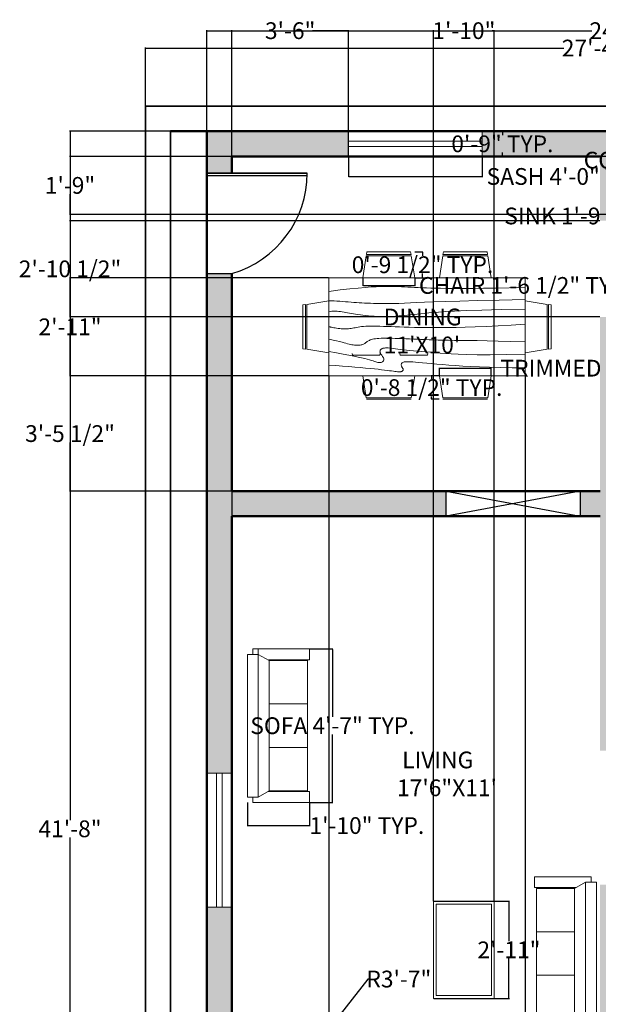
# Model space of a CAD drawing. Units: inches. Extents: x 3398 to 3816, y 15195 to 15771.
# Tile 7 of 10: x 3398 to 3606, y 15418 to 15771. Entities that reach past the tile are written whole.
import ezdxf

# ---------------------------------------------------------------- set-up
doc = ezdxf.new("R2010")
doc.units = ezdxf.units.IN
doc.header["$MEASUREMENT"] = 0
for name, color, linetype, lineweight in [('A-ANNO-DIMS', 2, 'Continuous', 18), ('A-AREA-IDEN', 7, 'Continuous', 25), ('A-DOOR', 3, 'Continuous', 25), ('A-FURN', 8, 'Continuous', 18), ('A-GLAZ', 4, 'Continuous', 18), ('A-WALL', 7, 'Continuous', 50), ('A-WALL-OPEN', 7, 'Continuous', 25), ('A-WALL-PATT', 252, 'Continuous', 13), ('C-PROP', 7, 'Continuous', 35)]:
    doc.layers.add(name, color=color, linetype=linetype, lineweight=lineweight)
doc.styles.get("Standard").update_dxf_attribs({"font": 'arial.ttf'})
doc.dimstyles.get("Standard").update_dxf_attribs({"dimtxt": 6, "dimasz": 0.18, "dimexe": 0.18, "dimexo": 0.0625, "dimgap": 0.09, "dimtad": 0, "dimtih": 1, "dimtoh": 1, "dimdec": 1, "dimzin": 0, "dimdsep": 46, "dimlunit": 3, "dimtxsty": 'Standard', "dimcen": 0.09, "dimadec": 0, "dimazin": 0, "dimtfac": 1, "dimtdec": 1, "dimtofl": 0, "dimtmove": 0, "dimatfit": 3, "dimfxl": 1, "dimtolj": 1, "dimtzin": 0, "dimarcsym": 0})

# ---------------------------------------------------------------- blocks, each defined once
blk = doc.blocks.new('*D4')
at = {"layer": 'A-ANNO-DIMS', "color": 0, "lineweight": -2, "transparency": 16777216}
for p, q in [((3443.19, 15739.58), (3443.19, 15760.52)), ((3443.37, 15760.34), (3593.25, 15760.34)), ((3771.01, 15760.34), (3621.13, 15760.34)), ((3771.19, 15739.58), (3771.19, 15760.52))]:
    blk.add_line(p, q, dxfattribs=at)
at = {"layer": 'A-ANNO-DIMS', "color": 0, "transparency": 16777216}
for points in [[(3443.37, 15760.37), (3443.37, 15760.31), (3443.19, 15760.34)], [(3771.01, 15760.37), (3771.01, 15760.31), (3771.19, 15760.34)]]:
    blk.add_solid(points, dxfattribs=at)
at = {"layer": 'Defpoints', "color": 0, "transparency": 16777216}
for p in [(3771.19, 15760.34), (3443.19, 15739.52), (3771.19, 15739.52)]:
    blk.add_point(p, dxfattribs=at)
at = {"layer": 'A-ANNO-DIMS', "color": 0, "transparency": 16777216, "insert": (3607.19, 15760.34), "char_height": 6, "attachment_point": 5}
blk.add_mtext('\\A1;27\'-4.0"', dxfattribs=at)
blk = doc.blocks.new('SOFA-3-SEAT')
for p, q in [((0, 53.08), (0, 1.96)), ((3.92, 53.08), (0, 53.08)), ((1.96, 55.04), (22.23, 55.04)), ((1.96, 55.04), (1.96, 53.08)), ((3.92, 55.04), (3.92, 1.96)), ((3.92, 53.08), (7.85, 50.88)), ((22.23, 51.12), (22.23, 55.04)), ((7.54, 51.12), (22.23, 51.12)), ((21.58, 50.87), (7.85, 50.87)), ((21.58, 35.31), (7.85, 35.31)), ((21.58, 19.74), (7.85, 19.74)), ((7.85, 4.17), (3.92, 1.96)), ((7.29, 3.92), (22.23, 3.92)), ((22.23, 3.92), (22.23, 0)), ((3.92, 1.96), (0, 1.96)), ((1.96, 1.96), (1.96, 0)), ((1.96, 0), (22.23, 0))]:
    blk.add_line(p, q)
blk.add_lwpolyline([(7.85, 50.88), (7.85, 4.17), (21.58, 4.17), (21.58, 50.87)])
blk = doc.blocks.new('WINDOW-SASH-48IN')
for p, q in [((48, 9), (0, 9)), ((48, 5.5), (0, 5.5)), ((0, 3.5), (48, 3.5)), ((0, 0), (48, 0))]:
    blk.add_line(p, q)
blk = doc.blocks.new('CHAIR-DINING')
for p, q in [((0, 0), (1.22, 7.83)), ((17.33, 7.83), (1.22, 7.83)), ((1.3, 8.32), (1.45, 9.3)), ((1.3, 8.32), (17.26, 8.32)), ((17.11, 9.3), (1.45, 9.3)), ((17.11, 9.3), (17.26, 8.32)), ((17.34, 7.83), (18.56, 0))]:
    blk.add_line(p, q)
blk = doc.blocks.new('CHAIR-DINING-TRIMMED')
for p, q in [((0, 8.32), (1.22, 0.49)), ((17.34, 0.49), (18.56, 8.32)), ((17.33, 0.49), (1.22, 0.49)), ((1.3, 0), (17.26, 0))]:
    blk.add_line(p, q)
blk = doc.blocks.new('*D14')
at = {"layer": 'A-ANNO-DIMS', "color": 0, "lineweight": -2, "transparency": 16777216}
for p, q in [((3515.96, 15721.46), (3515.96, 15714.14)), ((3563.96, 15721.46), (3563.96, 15714.14)), ((3516.14, 15714.32), (3563.78, 15714.32)), ((3563.96, 15714.32), (3564.14, 15714.32))]:
    blk.add_line(p, q, dxfattribs=at)
at = {"layer": 'A-ANNO-DIMS', "color": 0, "transparency": 16777216}
for points in [[(3516.14, 15714.35), (3516.14, 15714.29), (3515.96, 15714.32)], [(3563.78, 15714.35), (3563.78, 15714.29), (3563.96, 15714.32)]]:
    blk.add_solid(points, dxfattribs=at)
at = {"layer": 'Defpoints', "color": 0, "transparency": 16777216}
for p in [(3515.96, 15721.52), (3563.96, 15721.52), (3563.96, 15714.32)]:
    blk.add_point(p, dxfattribs=at)
at = {"layer": 'A-ANNO-DIMS', "color": 0, "transparency": 16777216, "insert": (3595.08, 15714.32), "char_height": 6, "attachment_point": 5}
blk.add_mtext('\\A1;SASH 4\'-0" TYP.', dxfattribs=at)
blk = doc.blocks.new('*D15')
at = {"layer": 'A-ANNO-DIMS', "color": 0, "lineweight": -2, "transparency": 16777216}
for p, q in [((3564.02, 15730.52), (3571.34, 15730.52)), ((3571.16, 15730.34), (3571.16, 15729.17)), ((3564.02, 15721.52), (3571.34, 15721.52)), ((3571.16, 15721.7), (3571.16, 15722.87))]:
    blk.add_line(p, q, dxfattribs=at)
at = {"layer": 'A-ANNO-DIMS', "color": 0, "transparency": 16777216}
for points in [[(3571.13, 15730.34), (3571.19, 15730.34), (3571.16, 15730.52)], [(3571.13, 15721.7), (3571.19, 15721.7), (3571.16, 15721.52)]]:
    blk.add_solid(points, dxfattribs=at)
at = {"layer": 'Defpoints', "color": 0, "transparency": 16777216}
for p in [(3563.96, 15730.52), (3571.16, 15730.52), (3563.96, 15721.52)]:
    blk.add_point(p, dxfattribs=at)
at = {"layer": 'A-ANNO-DIMS', "color": 0, "transparency": 16777216, "insert": (3571.16, 15726.02), "char_height": 6, "attachment_point": 5}
blk.add_mtext('\\A1;0\'-9" TYP.', dxfattribs=at)
blk = doc.blocks.new('*D16')
at = {"layer": 'A-ANNO-DIMS', "color": 0, "lineweight": -2, "transparency": 16777216}
for p, q in [((3521.16, 15677.98), (3521.16, 15675.08)), ((3521.34, 15675.26), (3539.54, 15675.26)), ((3539.72, 15677.98), (3539.72, 15675.08)), ((3539.72, 15675.26), (3539.9, 15675.26))]:
    blk.add_line(p, q, dxfattribs=at)
at = {"layer": 'A-ANNO-DIMS', "color": 0, "transparency": 16777216}
for points in [[(3521.34, 15675.29), (3521.34, 15675.23), (3521.16, 15675.26)], [(3539.54, 15675.29), (3539.54, 15675.23), (3539.72, 15675.26)]]:
    blk.add_solid(points, dxfattribs=at)
at = {"layer": 'Defpoints', "color": 0, "transparency": 16777216}
for p in [(3521.16, 15678.04), (3539.72, 15678.04), (3539.72, 15675.26)]:
    blk.add_point(p, dxfattribs=at)
at = {"layer": 'A-ANNO-DIMS', "color": 0, "transparency": 16777216, "insert": (3579.44, 15675.26), "char_height": 6, "attachment_point": 5}
blk.add_mtext('\\A1;CHAIR 1\'-6 1/2" TYP.', dxfattribs=at)
blk = doc.blocks.new('*D17')
at = {"layer": 'A-ANNO-DIMS', "color": 0, "lineweight": -2, "transparency": 16777216}
for p, q in [((3539.79, 15687.34), (3542.69, 15687.34)), ((3542.51, 15687.16), (3542.51, 15685.88)), ((3542.51, 15678.22), (3542.51, 15679.5)), ((3539.79, 15678.04), (3542.69, 15678.04))]:
    blk.add_line(p, q, dxfattribs=at)
at = {"layer": 'A-ANNO-DIMS', "color": 0, "transparency": 16777216}
for points in [[(3542.48, 15687.16), (3542.54, 15687.16), (3542.51, 15687.34)], [(3542.48, 15678.22), (3542.54, 15678.22), (3542.51, 15678.04)]]:
    blk.add_solid(points, dxfattribs=at)
at = {"layer": 'Defpoints', "color": 0, "transparency": 16777216}
for p in [(3539.72, 15687.34), (3542.51, 15687.34), (3539.72, 15678.04)]:
    blk.add_point(p, dxfattribs=at)
at = {"layer": 'A-ANNO-DIMS', "color": 0, "transparency": 16777216, "insert": (3542.51, 15682.69), "char_height": 6, "attachment_point": 5}
blk.add_mtext('\\A1;0\'-9 1/2" TYP.', dxfattribs=at)
blk = doc.blocks.new('*D18')
at = {"layer": 'A-ANNO-DIMS', "color": 0, "lineweight": -2, "transparency": 16777216}
for p, q in [((3548.56, 15642.88), (3548.56, 15645.79)), ((3548.74, 15645.61), (3566.94, 15645.61)), ((3567.12, 15642.88), (3567.12, 15645.79)), ((3567.12, 15645.61), (3567.3, 15645.61))]:
    blk.add_line(p, q, dxfattribs=at)
at = {"layer": 'A-ANNO-DIMS', "color": 0, "transparency": 16777216}
for points in [[(3548.74, 15645.64), (3548.74, 15645.58), (3548.56, 15645.61)], [(3566.94, 15645.64), (3566.94, 15645.58), (3567.12, 15645.61)]]:
    blk.add_solid(points, dxfattribs=at)
at = {"layer": 'Defpoints', "color": 0, "transparency": 16777216}
for p in [(3567.12, 15645.61), (3548.56, 15642.82), (3567.12, 15642.82)]:
    blk.add_point(p, dxfattribs=at)
at = {"layer": 'A-ANNO-DIMS', "color": 0, "transparency": 16777216, "insert": (3627.67, 15645.61), "char_height": 6, "attachment_point": 5}
blk.add_mtext('\\A1;TRIMMED CHAIR 1\'-6 1/2" TYP.', dxfattribs=at)
blk = doc.blocks.new('*D19')
at = {"layer": 'A-ANNO-DIMS', "color": 0, "lineweight": -2, "transparency": 16777216}
for p, q in [((3548.5, 15642.82), (3545.6, 15642.82)), ((3545.78, 15642.64), (3545.78, 15641.85)), ((3548.5, 15634.5), (3545.6, 15634.5)), ((3545.78, 15634.68), (3545.78, 15635.47))]:
    blk.add_line(p, q, dxfattribs=at)
at = {"layer": 'A-ANNO-DIMS', "color": 0, "transparency": 16777216}
for points in [[(3545.75, 15642.64), (3545.81, 15642.64), (3545.78, 15642.82)], [(3545.75, 15634.68), (3545.81, 15634.68), (3545.78, 15634.5)]]:
    blk.add_solid(points, dxfattribs=at)
at = {"layer": 'Defpoints', "color": 0, "transparency": 16777216}
for p in [(3545.78, 15642.82), (3548.56, 15642.82), (3548.56, 15634.5)]:
    blk.add_point(p, dxfattribs=at)
at = {"layer": 'A-ANNO-DIMS', "color": 0, "transparency": 16777216, "insert": (3545.78, 15638.66), "char_height": 6, "attachment_point": 5}
blk.add_mtext('\\A1;0\'-8 1/2" TYP.', dxfattribs=at)
blk = doc.blocks.new('*D20')
at = {"layer": 'A-ANNO-DIMS', "color": 0, "lineweight": -2, "transparency": 16777216}
for p, q in [((3502.02, 15545), (3510.4, 15545)), ((3510.22, 15544.82), (3510.22, 15520.67)), ((3510.22, 15490.13), (3510.22, 15514.28)), ((3502.02, 15489.95), (3510.4, 15489.95))]:
    blk.add_line(p, q, dxfattribs=at)
at = {"layer": 'A-ANNO-DIMS', "color": 0, "transparency": 16777216}
for points in [[(3510.19, 15544.82), (3510.25, 15544.82), (3510.22, 15545)], [(3510.19, 15490.13), (3510.25, 15490.13), (3510.22, 15489.95)]]:
    blk.add_solid(points, dxfattribs=at)
at = {"layer": 'Defpoints', "color": 0, "transparency": 16777216}
for p in [(3501.96, 15545), (3510.22, 15545), (3501.96, 15489.95)]:
    blk.add_point(p, dxfattribs=at)
at = {"layer": 'A-ANNO-DIMS', "color": 0, "transparency": 16777216, "insert": (3510.22, 15517.47), "char_height": 6, "attachment_point": 5}
blk.add_mtext('\\A1;SOFA 4\'-7" TYP.', dxfattribs=at)
blk = doc.blocks.new('*D21')
at = {"layer": 'A-ANNO-DIMS', "color": 0, "lineweight": -2, "transparency": 16777216}
for p, q in [((3479.73, 15489.89), (3479.73, 15481.51)), ((3501.96, 15489.89), (3501.96, 15481.51)), ((3479.91, 15481.69), (3501.78, 15481.69)), ((3501.96, 15481.69), (3502.14, 15481.69))]:
    blk.add_line(p, q, dxfattribs=at)
at = {"layer": 'A-ANNO-DIMS', "color": 0, "transparency": 16777216}
for points in [[(3479.91, 15481.72), (3479.91, 15481.66), (3479.73, 15481.69)], [(3501.78, 15481.72), (3501.78, 15481.66), (3501.96, 15481.69)]]:
    blk.add_solid(points, dxfattribs=at)
at = {"layer": 'Defpoints', "color": 0, "transparency": 16777216}
for p in [(3479.73, 15489.95), (3501.96, 15489.95), (3501.96, 15481.69)]:
    blk.add_point(p, dxfattribs=at)
at = {"layer": 'A-ANNO-DIMS', "color": 0, "transparency": 16777216, "insert": (3522.57, 15481.69), "char_height": 6, "attachment_point": 5}
blk.add_mtext('\\A1;1\'-10" TYP.', dxfattribs=at)
blk = doc.blocks.new('*D30')
at = {"layer": 'A-ANNO-DIMS', "color": 0, "lineweight": -2, "transparency": 16777216}
for p, q in [((3660.03, 15720.16), (3659.85, 15720.16)), ((3660.03, 15717.39), (3660.03, 15720.34)), ((3678.72, 15720.16), (3660.21, 15720.16)), ((3678.9, 15717.39), (3678.9, 15720.34))]:
    blk.add_line(p, q, dxfattribs=at)
at = {"layer": 'A-ANNO-DIMS', "color": 0, "transparency": 16777216}
for points in [[(3660.21, 15720.19), (3660.21, 15720.13), (3660.03, 15720.16)], [(3678.72, 15720.19), (3678.72, 15720.13), (3678.9, 15720.16)]]:
    blk.add_solid(points, dxfattribs=at)
at = {"layer": 'Defpoints', "color": 0, "transparency": 16777216}
for p in [(3660.03, 15720.16), (3660.03, 15717.33), (3678.9, 15717.33)]:
    blk.add_point(p, dxfattribs=at)
at = {"layer": 'A-ANNO-DIMS', "color": 0, "transparency": 16777216, "insert": (3629.7, 15720.16), "char_height": 6, "attachment_point": 5}
blk.add_mtext('\\A1;COOKTOP 1\'-7"', dxfattribs=at)
blk = doc.blocks.new('*D32')
at = {"layer": 'A-ANNO-DIMS', "color": 0, "lineweight": -2, "transparency": 16777216}
for p, q in [((3624.27, 15700.17), (3624.09, 15700.17)), ((3624.27, 15703.37), (3624.27, 15699.99)), ((3645.8, 15700.17), (3624.45, 15700.17)), ((3645.98, 15703.37), (3645.98, 15699.99))]:
    blk.add_line(p, q, dxfattribs=at)
at = {"layer": 'A-ANNO-DIMS', "color": 0, "transparency": 16777216}
for points in [[(3624.45, 15700.2), (3624.45, 15700.14), (3624.27, 15700.17)], [(3645.8, 15700.2), (3645.8, 15700.14), (3645.98, 15700.17)]]:
    blk.add_solid(points, dxfattribs=at)
at = {"layer": 'Defpoints', "color": 0, "transparency": 16777216}
for p in [(3624.27, 15703.43), (3624.27, 15700.17), (3645.98, 15703.43)]:
    blk.add_point(p, dxfattribs=at)
at = {"layer": 'A-ANNO-DIMS', "color": 0, "transparency": 16777216, "insert": (3598.1, 15700.17), "char_height": 6, "attachment_point": 5}
blk.add_mtext('\\A1;SINK 1\'-9 1/2"', dxfattribs=at)
blk = doc.blocks.new('*D36')
at = {"layer": 'A-ANNO-DIMS', "color": 0, "lineweight": -2, "transparency": 16777216}
for p, q in [((3465.19, 15730.58), (3465.19, 15766.75)), ((3465.37, 15766.57), (3603.24, 15766.57)), ((3762.01, 15766.57), (3624.14, 15766.57)), ((3762.19, 15730.58), (3762.19, 15766.75))]:
    blk.add_line(p, q, dxfattribs=at)
at = {"layer": 'A-ANNO-DIMS', "color": 0, "transparency": 16777216}
for points in [[(3465.37, 15766.6), (3465.37, 15766.54), (3465.19, 15766.57)], [(3762.01, 15766.6), (3762.01, 15766.54), (3762.19, 15766.57)]]:
    blk.add_solid(points, dxfattribs=at)
at = {"layer": 'Defpoints', "color": 0, "transparency": 16777216}
for p in [(3762.19, 15766.57), (3465.19, 15730.52), (3762.19, 15730.52)]:
    blk.add_point(p, dxfattribs=at)
at = {"layer": 'A-ANNO-DIMS', "color": 0, "transparency": 16777216, "insert": (3613.69, 15766.57), "char_height": 6, "attachment_point": 5}
blk.add_mtext('\\A1;24\'-9"', dxfattribs=at)
blk = doc.blocks.new('*D38')
at = {"layer": 'A-ANNO-DIMS', "color": 0, "lineweight": -2, "transparency": 16777216}
for p, q in [((3465.13, 15730.52), (3415.96, 15730.52)), ((3416.14, 15730.34), (3416.14, 15483.67)), ((3416.14, 15230.7), (3416.14, 15477.37)), ((3465.74, 15230.52), (3415.96, 15230.52))]:
    blk.add_line(p, q, dxfattribs=at)
at = {"layer": 'A-ANNO-DIMS', "color": 0, "transparency": 16777216}
for points in [[(3416.11, 15730.34), (3416.17, 15730.34), (3416.14, 15730.52)], [(3416.11, 15230.7), (3416.17, 15230.7), (3416.14, 15230.52)]]:
    blk.add_solid(points, dxfattribs=at)
at = {"layer": 'Defpoints', "color": 0, "transparency": 16777216}
for p in [(3416.14, 15730.52), (3465.19, 15730.52), (3465.8, 15230.52)]:
    blk.add_point(p, dxfattribs=at)
at = {"layer": 'A-ANNO-DIMS', "color": 0, "transparency": 16777216, "insert": (3416.14, 15480.52), "char_height": 6, "attachment_point": 5}
blk.add_mtext('\\A1;41\'-8"', dxfattribs=at)
blk = doc.blocks.new('*D44')
at = {"layer": 'A-ANNO-DIMS', "color": 0, "lineweight": -2, "transparency": 16777216}
for p, q in [((3508.92, 15642.76), (3508.92, 15203.29)), ((3579.37, 15642.76), (3579.37, 15203.29)), ((3509.1, 15203.47), (3526.76, 15203.47)), ((3579.19, 15203.47), (3561.53, 15203.47))]:
    blk.add_line(p, q, dxfattribs=at)
at = {"layer": 'A-ANNO-DIMS', "color": 0, "transparency": 16777216}
for points in [[(3509.1, 15203.5), (3509.1, 15203.44), (3508.92, 15203.47)], [(3579.19, 15203.5), (3579.19, 15203.44), (3579.37, 15203.47)]]:
    blk.add_solid(points, dxfattribs=at)
at = {"layer": 'Defpoints', "color": 0, "transparency": 16777216}
for p in [(3508.92, 15642.82), (3579.37, 15642.82), (3579.37, 15203.47)]:
    blk.add_point(p, dxfattribs=at)
at = {"layer": 'A-ANNO-DIMS', "color": 0, "transparency": 16777216, "insert": (3544.14, 15203.47), "char_height": 6, "attachment_point": 5}
blk.add_mtext('\\A1;5\'-10 1/2"', dxfattribs=at)
blk = doc.blocks.new('*D45')
at = {"layer": 'A-ANNO-DIMS', "color": 0, "lineweight": -2, "transparency": 16777216}
for p, q in [((3508.86, 15678.04), (3415.96, 15678.04)), ((3416.14, 15677.86), (3416.14, 15663.53)), ((3416.14, 15643), (3416.14, 15657.33)), ((3508.86, 15642.82), (3415.96, 15642.82))]:
    blk.add_line(p, q, dxfattribs=at)
at = {"layer": 'A-ANNO-DIMS', "color": 0, "transparency": 16777216}
for points in [[(3416.11, 15677.86), (3416.17, 15677.86), (3416.14, 15678.04)], [(3416.11, 15643), (3416.17, 15643), (3416.14, 15642.82)]]:
    blk.add_solid(points, dxfattribs=at)
at = {"layer": 'Defpoints', "color": 0, "transparency": 16777216}
for p in [(3416.14, 15678.04), (3508.92, 15678.04), (3508.92, 15642.82)]:
    blk.add_point(p, dxfattribs=at)
at = {"layer": 'A-ANNO-DIMS', "color": 0, "transparency": 16777216, "insert": (3416.14, 15660.43), "char_height": 6, "attachment_point": 5}
blk.add_mtext('\\A1;2\'-11"', dxfattribs=at)
blk = doc.blocks.new('*D46')
at = {"layer": 'A-ANNO-DIMS', "color": 0, "lineweight": -2, "transparency": 16777216}
for p, q in [((3606.13, 15698.45), (3415.96, 15698.45)), ((3416.14, 15698.27), (3416.14, 15684.4)), ((3416.14, 15664.15), (3416.14, 15678.02)), ((3606.13, 15663.97), (3415.96, 15663.97))]:
    blk.add_line(p, q, dxfattribs=at)
at = {"layer": 'A-ANNO-DIMS', "color": 0, "transparency": 16777216}
for points in [[(3416.11, 15698.27), (3416.17, 15698.27), (3416.14, 15698.45)], [(3416.11, 15664.15), (3416.17, 15664.15), (3416.14, 15663.97)]]:
    blk.add_solid(points, dxfattribs=at)
at = {"layer": 'Defpoints', "color": 0, "transparency": 16777216}
for p in [(3416.14, 15698.45), (3606.19, 15698.45), (3606.19, 15663.97)]:
    blk.add_point(p, dxfattribs=at)
at = {"layer": 'A-ANNO-DIMS', "color": 0, "transparency": 16777216, "insert": (3416.14, 15681.21), "char_height": 6, "attachment_point": 5}
blk.add_mtext('\\A1;2\'-10 1/2"', dxfattribs=at)
blk = doc.blocks.new('*D49')
at = {"layer": 'A-ANNO-DIMS', "color": 0, "lineweight": -2, "transparency": 16777216}
for p, q in [((3700.63, 15721.52), (3415.96, 15721.52)), ((3416.14, 15721.34), (3416.14, 15714.27)), ((3416.14, 15700.89), (3416.14, 15707.96)), ((3700.63, 15700.71), (3415.96, 15700.71))]:
    blk.add_line(p, q, dxfattribs=at)
at = {"layer": 'A-ANNO-DIMS', "color": 0, "transparency": 16777216}
for points in [[(3416.11, 15721.34), (3416.17, 15721.34), (3416.14, 15721.52)], [(3416.11, 15700.89), (3416.17, 15700.89), (3416.14, 15700.71)]]:
    blk.add_solid(points, dxfattribs=at)
at = {"layer": 'Defpoints', "color": 0, "transparency": 16777216}
for p in [(3416.14, 15721.52), (3700.69, 15721.52), (3700.69, 15700.71)]:
    blk.add_point(p, dxfattribs=at)
at = {"layer": 'A-ANNO-DIMS', "color": 0, "transparency": 16777216, "insert": (3416.14, 15711.12), "char_height": 6, "attachment_point": 5}
blk.add_mtext('\\A1;1\'-9"', dxfattribs=at)
blk = doc.blocks.new('*D50')
at = {"layer": 'A-ANNO-DIMS', "color": 0, "lineweight": -2, "transparency": 16777216}
for p, q in [((3546.47, 15454.62), (3546.47, 15766.75)), ((3546.65, 15766.57), (3547.24, 15766.57)), ((3568.05, 15766.57), (3567.46, 15766.57)), ((3568.23, 15454.62), (3568.23, 15766.75))]:
    blk.add_line(p, q, dxfattribs=at)
at = {"layer": 'A-ANNO-DIMS', "color": 0, "transparency": 16777216}
for points in [[(3546.65, 15766.6), (3546.65, 15766.54), (3546.47, 15766.57)], [(3568.05, 15766.6), (3568.05, 15766.54), (3568.23, 15766.57)]]:
    blk.add_solid(points, dxfattribs=at)
at = {"layer": 'Defpoints', "color": 0, "transparency": 16777216}
for p in [(3568.23, 15766.57), (3546.47, 15454.56), (3568.23, 15454.56)]:
    blk.add_point(p, dxfattribs=at)
at = {"layer": 'A-ANNO-DIMS', "color": 0, "transparency": 16777216, "insert": (3557.35, 15766.57), "char_height": 6, "attachment_point": 5}
blk.add_mtext('\\A1;1\'-10"', dxfattribs=at)
blk = doc.blocks.new('*D51')
at = {"layer": 'A-ANNO-DIMS', "color": 0, "lineweight": -2, "transparency": 16777216}
for p, q in [((3546.53, 15454.56), (3573.7, 15454.56)), ((3573.52, 15454.38), (3573.52, 15440.24)), ((3573.52, 15419.9), (3573.52, 15434.04)), ((3546.53, 15419.72), (3573.7, 15419.72))]:
    blk.add_line(p, q, dxfattribs=at)
at = {"layer": 'A-ANNO-DIMS', "color": 0, "transparency": 16777216}
for points in [[(3573.49, 15454.38), (3573.55, 15454.38), (3573.52, 15454.56)], [(3573.49, 15419.9), (3573.55, 15419.9), (3573.52, 15419.72)]]:
    blk.add_solid(points, dxfattribs=at)
at = {"layer": 'Defpoints', "color": 0, "transparency": 16777216}
for p in [(3546.47, 15454.56), (3546.47, 15419.72), (3573.52, 15419.72)]:
    blk.add_point(p, dxfattribs=at)
at = {"layer": 'A-ANNO-DIMS', "color": 0, "transparency": 16777216, "insert": (3573.52, 15437.14), "char_height": 6, "attachment_point": 5}
blk.add_mtext('\\A1;2\'-11"', dxfattribs=at)
blk = doc.blocks.new('*D52')
at = {"layer": 'A-ANNO-DIMS', "color": 0, "lineweight": -2, "transparency": 16777216}
for p, q in [((3474.19, 15721.58), (3474.19, 15766.75)), ((3474.37, 15766.57), (3487.01, 15766.57)), ((3515.78, 15766.57), (3503.14, 15766.57)), ((3515.96, 15721.58), (3515.96, 15766.75))]:
    blk.add_line(p, q, dxfattribs=at)
at = {"layer": 'A-ANNO-DIMS', "color": 0, "transparency": 16777216}
for points in [[(3474.37, 15766.6), (3474.37, 15766.54), (3474.19, 15766.57)], [(3515.78, 15766.6), (3515.78, 15766.54), (3515.96, 15766.57)]]:
    blk.add_solid(points, dxfattribs=at)
at = {"layer": 'Defpoints', "color": 0, "transparency": 16777216}
for p in [(3515.96, 15766.57), (3474.19, 15721.52), (3515.96, 15721.52)]:
    blk.add_point(p, dxfattribs=at)
at = {"layer": 'A-ANNO-DIMS', "color": 0, "transparency": 16777216, "insert": (3495.07, 15766.57), "char_height": 6, "attachment_point": 5}
blk.add_mtext('\\A1;3\'-6"', dxfattribs=at)
blk = doc.blocks.new('*D53')
at = {"layer": 'A-ANNO-DIMS', "color": 0, "lineweight": -2, "transparency": 16777216}
for p, q in [((3508.92, 15642.76), (3508.92, 15203.29)), ((3474.19, 15601.46), (3474.19, 15203.29)), ((3474.37, 15203.47), (3508.74, 15203.47)), ((3508.92, 15203.47), (3509.1, 15203.47))]:
    blk.add_line(p, q, dxfattribs=at)
at = {"layer": 'A-ANNO-DIMS', "color": 0, "transparency": 16777216}
for points in [[(3474.37, 15203.5), (3474.37, 15203.44), (3474.19, 15203.47)], [(3508.74, 15203.5), (3508.74, 15203.44), (3508.92, 15203.47)]]:
    blk.add_solid(points, dxfattribs=at)
at = {"layer": 'Defpoints', "color": 0, "transparency": 16777216}
for p in [(3508.92, 15642.82), (3474.19, 15601.52), (3508.92, 15203.47)]:
    blk.add_point(p, dxfattribs=at)
at = {"layer": 'A-ANNO-DIMS', "color": 0, "transparency": 16777216, "insert": (3526.54, 15203.47), "char_height": 6, "attachment_point": 5}
blk.add_mtext('\\A1;2\'-10 1/2"', dxfattribs=at)
blk = doc.blocks.new('*D54')
at = {"layer": 'A-ANNO-DIMS', "color": 0, "lineweight": -2, "transparency": 16777216}
for p, q in [((3508.86, 15642.82), (3415.96, 15642.82)), ((3416.14, 15642.64), (3416.14, 15625.36)), ((3416.14, 15601.7), (3416.14, 15618.98)), ((3474.13, 15601.52), (3415.96, 15601.52))]:
    blk.add_line(p, q, dxfattribs=at)
at = {"layer": 'A-ANNO-DIMS', "color": 0, "transparency": 16777216}
for points in [[(3416.11, 15642.64), (3416.17, 15642.64), (3416.14, 15642.82)], [(3416.11, 15601.7), (3416.17, 15601.7), (3416.14, 15601.52)]]:
    blk.add_solid(points, dxfattribs=at)
at = {"layer": 'Defpoints', "color": 0, "transparency": 16777216}
for p in [(3508.92, 15642.82), (3416.14, 15601.52), (3474.19, 15601.52)]:
    blk.add_point(p, dxfattribs=at)
at = {"layer": 'A-ANNO-DIMS', "color": 0, "transparency": 16777216, "insert": (3416.14, 15622.17), "char_height": 6, "attachment_point": 5}
blk.add_mtext('\\A1;3\'-5 1/2"', dxfattribs=at)
blk = doc.blocks.new('*D55')
at = {"layer": 'A-ANNO-DIMS', "color": 0, "lineweight": -2, "transparency": 16777216}
for p, q in [((3522.92, 15426.68), (3507.01, 15406.43)), ((3523.1, 15426.68), (3522.92, 15426.68)), ((3480.1, 15372.29), (3480.28, 15372.29)), ((3480.19, 15372.2), (3480.19, 15372.38))]:
    blk.add_line(p, q, dxfattribs=at)
at = {"layer": 'A-ANNO-DIMS', "color": 0, "transparency": 16777216}
blk.add_solid([(3506.98, 15406.44), (3507.03, 15406.41), (3506.9, 15406.28)], dxfattribs=at)
at = {"layer": 'Defpoints', "color": 0, "transparency": 16777216}
for p in [(3506.9, 15406.28), (3480.19, 15372.29)]:
    blk.add_point(p, dxfattribs=at)
at = {"layer": 'A-ANNO-DIMS', "color": 0, "transparency": 16777216, "insert": (3534.04, 15426.68), "char_height": 6, "attachment_point": 5}
blk.add_mtext('\\A1;R3\'-7"', dxfattribs=at)

msp = doc.modelspace()

# ---------------------------------------------------------------- hatches: boundary and pattern name
at = {"layer": 'A-WALL-PATT'}
h = msp.add_hatch(color=256, dxfattribs=at)
h.dxf.hatch_style = 1
h.paths.add_polyline_path([(3515.96, 15730.52), (3465.19, 15730.52), (3465.19, 15715.52), (3474.19, 15715.52), (3474.19, 15721.52), (3515.96, 15721.52)])
h.paths.add_polyline_path([(3719.81, 15730.52), (3675.76, 15730.52), (3675.76, 15721.52), (3700.69, 15721.52), (3700.69, 15637.52), (3610.69, 15637.52), (3610.69, 15663.97), (3606.19, 15663.97), (3606.19, 15601.52), (3599.08, 15601.52), (3599.08, 15592.52), (3606.19, 15592.52), (3606.19, 15508.52), (3616.69, 15508.52), (3616.69, 15513.02), (3610.69, 15513.02), (3610.69, 15633.02), (3708.19, 15633.02), (3708.19, 15637.52), (3705.19, 15637.52), (3705.19, 15721.52), (3719.81, 15721.52)])
h.paths.add_polyline_path([(3762.19, 15730.52), (3743.77, 15730.52), (3743.77, 15721.52), (3753.19, 15721.52), (3753.19, 15637.52), (3732.19, 15637.52), (3732.19, 15633.02), (3753.19, 15633.02), (3753.19, 15597.39), (3762.19, 15597.39)])
h.paths.add_polyline_path([(3762.19, 15549.39), (3753.19, 15549.39), (3753.19, 15513.02), (3652.69, 15513.02), (3652.69, 15508.52), (3664.69, 15508.52), (3664.69, 15460.52), (3652.69, 15460.52), (3652.69, 15456.02), (3672.19, 15456.02), (3672.19, 15460.52), (3669.19, 15460.52), (3669.19, 15508.52), (3753.19, 15508.52), (3753.19, 15497.51), (3762.19, 15497.51)])
h.paths.add_polyline_path([(3762.19, 15473.48), (3753.19, 15473.48), (3753.19, 15460.52), (3696.19, 15460.52), (3696.19, 15456.02), (3753.19, 15456.02), (3753.19, 15414.25), (3762.19, 15414.25)])
h.paths.add_polyline_path([(3762.19, 15366.28), (3753.19, 15366.28), (3753.19, 15324.02), (3610.69, 15324.02), (3610.69, 15456.02), (3616.69, 15456.02), (3616.69, 15460.52), (3610.69, 15460.52), (3606.19, 15460.52), (3606.19, 15382.52), (3587.73, 15382.52), (3587.73, 15373.52), (3606.19, 15373.52), (3606.19, 15315.02), (3762.19, 15315.02)])
h.paths.add_polyline_path([(3539.73, 15382.52), (3522.19, 15382.52), (3522.19, 15373.52), (3539.73, 15373.52)])
h.paths.add_polyline_path([(3480.19, 15382.52), (3474.19, 15382.52), (3474.19, 15452.47), (3465.19, 15452.47), (3465.19, 15373.52), (3480.19, 15373.52)])
h.paths.add_polyline_path([(3551.04, 15601.52), (3474.19, 15601.52), (3474.19, 15679.52), (3465.19, 15679.52), (3465.19, 15500.47), (3474.19, 15500.47), (3474.19, 15592.52), (3551.04, 15592.52)])
h = msp.add_hatch(color=256, dxfattribs=at)
h.dxf.hatch_style = 1
h.paths.add_polyline_path([(3610.69, 15721.52), (3639.76, 15721.52), (3639.76, 15730.52), (3563.96, 15730.52), (3563.96, 15721.52), (3606.19, 15721.52), (3606.19, 15700.71), (3606.19, 15698.45), (3610.7, 15698.45), (3610.7, 15700.71), (3610.69, 15700.71)])

# ---------------------------------------------------------------- linework, layer by layer
at = {"layer": 'A-DOOR'}
for p, q in [((3465.19, 15721.52), (3465.19, 15715.52)), ((3465.19, 15715.52), (3501.19, 15715.52)), ((3501.19, 15715.52), (3465.19, 15715.52)), ((3465.19, 15715.52), (3465.19, 15679.52)), ((3501.19, 15714.52), (3465.19, 15714.52)), ((3465.19, 15679.52), (3474.19, 15679.52))]:
    msp.add_line(p, q, dxfattribs=at)
msp.add_arc((3463.69, 15715.52), 37.5, 286.2602, 0, dxfattribs=at)
at = {"layer": 'A-FURN'}
for p, q in [((3579.37, 15678.04), (3508.92, 15678.04)), ((3508.92, 15678.04), (3508.92, 15642.82)), ((3579.37, 15642.82), (3579.37, 15678.04)), ((3517.36, 15650.9), (3517.46, 15650.29)), ((3527.22, 15650.29), (3527.31, 15650.9)), ((3534.44, 15650.9), (3534.54, 15650.29)), ((3544.3, 15650.29), (3544.39, 15650.9)), ((3527.22, 15650.29), (3517.46, 15650.29)), ((3544.3, 15650.29), (3534.54, 15650.29)), ((3508.92, 15642.82), (3579.37, 15642.82))]:
    msp.add_line(p, q, dxfattribs=at)
for points in [[(3579.37, 15674.62), (3573.58, 15674.46), (3568.64, 15674.34), (3564.43, 15674.25), (3560.85, 15674.2), (3557.81, 15674.18), (3555.2, 15674.17), (3552.92, 15674.19), (3550.87, 15674.21), (3548.96, 15674.25), (3547.17, 15674.29), (3545.48, 15674.33), (3543.9, 15674.38), (3542.42, 15674.44), (3541.01, 15674.5), (3539.69, 15674.56), (3538.43, 15674.62), (3537.24, 15674.68), (3536.09, 15674.74), (3534.95, 15674.79), (3533.82, 15674.84), (3532.68, 15674.87), (3531.49, 15674.9), (3530.25, 15674.91), (3528.94, 15674.9), (3527.52, 15674.88), (3525.93, 15674.82), (3524.1, 15674.72), (3521.97, 15674.56), (3519.46, 15674.34), (3516.49, 15674.04), (3513, 15673.65), (3508.92, 15673.15)], [(3579.37, 15670.22), (3569.98, 15670.03), (3562.21, 15669.85), (3555.87, 15669.68), (3550.74, 15669.51), (3546.61, 15669.36), (3543.28, 15669.22), (3540.54, 15669.1), (3538.19, 15668.99), (3536.04, 15668.91), (3534.06, 15668.85), (3532.23, 15668.81), (3530.55, 15668.79), (3528.99, 15668.78), (3527.55, 15668.79), (3526.22, 15668.8), (3524.98, 15668.83), (3523.83, 15668.86), (3522.75, 15668.91), (3521.72, 15668.95), (3520.73, 15669.01), (3519.77, 15669.07), (3518.82, 15669.13), (3517.87, 15669.2), (3516.91, 15669.28), (3515.92, 15669.36), (3514.9, 15669.43), (3513.88, 15669.51), (3512.85, 15669.58), (3511.83, 15669.64), (3510.83, 15669.69), (3509.86, 15669.72), (3508.92, 15669.73)], [(3579.37, 15666.79), (3570.74, 15666.61), (3563.79, 15666.43), (3558.3, 15666.25), (3554.03, 15666.07), (3550.77, 15665.89), (3548.29, 15665.73), (3546.36, 15665.56), (3544.75, 15665.41), (3543.29, 15665.26), (3541.92, 15665.11), (3540.63, 15664.98), (3539.42, 15664.85), (3538.27, 15664.74), (3537.17, 15664.63), (3536.11, 15664.52), (3535.09, 15664.43), (3534.09, 15664.34), (3533.11, 15664.26), (3532.14, 15664.19), (3531.18, 15664.14), (3530.21, 15664.1), (3529.24, 15664.08), (3528.26, 15664.08), (3527.26, 15664.1), (3526.25, 15664.14), (3525.21, 15664.2), (3524.18, 15664.28), (3523.16, 15664.38), (3522.15, 15664.48), (3521.18, 15664.59), (3520.24, 15664.71), (3519.36, 15664.83), (3518.53, 15664.96), (3517.75, 15665.08), (3517.03, 15665.2), (3516.33, 15665.32), (3515.67, 15665.44), (3515.03, 15665.55), (3514.4, 15665.66), (3513.77, 15665.77), (3513.14, 15665.88), (3512.51, 15665.97), (3511.89, 15666.04), (3511.27, 15666.08), (3510.66, 15666.09), (3510.06, 15666.05), (3509.48, 15665.96), (3508.92, 15665.81)], [(3579.37, 15661.41), (3574.27, 15661.08), (3569.6, 15660.81), (3565.33, 15660.59), (3561.42, 15660.43), (3557.84, 15660.31), (3554.56, 15660.22), (3551.56, 15660.17), (3548.79, 15660.15), (3546.23, 15660.14), (3543.86, 15660.15), (3541.67, 15660.18), (3539.63, 15660.21), (3537.73, 15660.26), (3535.96, 15660.31), (3534.3, 15660.37), (3532.73, 15660.43), (3531.24, 15660.49), (3529.82, 15660.55), (3528.49, 15660.6), (3527.23, 15660.65), (3526.06, 15660.68), (3524.96, 15660.7), (3523.95, 15660.7), (3523.02, 15660.68), (3522.18, 15660.63), (3521.41, 15660.57), (3520.7, 15660.5), (3520.06, 15660.41), (3519.46, 15660.32), (3518.91, 15660.22), (3518.39, 15660.12), (3517.89, 15660.02), (3517.41, 15659.94), (3516.93, 15659.86), (3516.46, 15659.79), (3515.99, 15659.74), (3515.51, 15659.7), (3515.02, 15659.68), (3514.51, 15659.68), (3513.97, 15659.7), (3513.41, 15659.74), (3512.83, 15659.8), (3512.26, 15659.87), (3511.7, 15659.95), (3511.17, 15660.04), (3510.69, 15660.12), (3510.27, 15660.2), (3509.94, 15660.27), (3509.69, 15660.32), (3509.52, 15660.36), (3509.4, 15660.39), (3509.32, 15660.41), (3509.25, 15660.42), (3509.18, 15660.43), (3509.07, 15660.43), (3508.92, 15660.43)], [(3579.37, 15655.05), (3574.2, 15655.21), (3569.65, 15655.33), (3565.66, 15655.42), (3562.17, 15655.49), (3559.11, 15655.53), (3556.42, 15655.57), (3554.04, 15655.59), (3551.89, 15655.62), (3549.92, 15655.66), (3548.11, 15655.7), (3546.43, 15655.74), (3544.87, 15655.79), (3543.39, 15655.85), (3541.97, 15655.91), (3540.6, 15655.97), (3539.25, 15656.03), (3537.91, 15656.09), (3536.57, 15656.15), (3535.27, 15656.2), (3533.99, 15656.25), (3532.76, 15656.29), (3531.59, 15656.33), (3530.49, 15656.35), (3529.47, 15656.35), (3528.53, 15656.35), (3527.69, 15656.32), (3526.92, 15656.29), (3526.24, 15656.23), (3525.62, 15656.16), (3525.07, 15656.08), (3524.59, 15655.98), (3524.17, 15655.87), (3523.79, 15655.74), (3523.47, 15655.59), (3523.18, 15655.44), (3522.92, 15655.28), (3522.69, 15655.12), (3522.47, 15654.96), (3522.26, 15654.8), (3522.05, 15654.64), (3521.83, 15654.49), (3521.6, 15654.35), (3521.36, 15654.23), (3521.1, 15654.11), (3520.82, 15654.01), (3520.52, 15653.93), (3520.2, 15653.87), (3519.84, 15653.83), (3519.46, 15653.81), (3519.05, 15653.81), (3518.62, 15653.83), (3518.16, 15653.88), (3517.69, 15653.94), (3517.2, 15654.02), (3516.69, 15654.12), (3516.18, 15654.23), (3515.65, 15654.37), (3515.08, 15654.52), (3514.43, 15654.69), (3513.68, 15654.89), (3512.78, 15655.12), (3511.72, 15655.38), (3510.44, 15655.68), (3508.92, 15656.03)], [(3579.37, 15650.65), (3572.49, 15650.51), (3566.82, 15650.45), (3562.17, 15650.45), (3558.4, 15650.51), (3555.34, 15650.62), (3552.83, 15650.75), (3550.71, 15650.9), (3548.83, 15651.05), (3547.05, 15651.2), (3545.34, 15651.35), (3543.71, 15651.48), (3542.16, 15651.62), (3540.69, 15651.74), (3539.31, 15651.87), (3538.01, 15651.99), (3536.8, 15652.11), (3535.69, 15652.24), (3534.66, 15652.36), (3533.72, 15652.47), (3532.86, 15652.57), (3532.08, 15652.67), (3531.38, 15652.75), (3530.75, 15652.81), (3530.2, 15652.85), (3529.71, 15652.87), (3529.29, 15652.87), (3528.92, 15652.84), (3528.61, 15652.8), (3528.34, 15652.73), (3528.11, 15652.65), (3527.92, 15652.56), (3527.75, 15652.44), (3527.61, 15652.31), (3527.5, 15652.17), (3527.4, 15652.01), (3527.34, 15651.85), (3527.3, 15651.68), (3527.28, 15651.5), (3527.3, 15651.32), (3527.35, 15651.14), (3527.42, 15650.95), (3527.52, 15650.77), (3527.64, 15650.59), (3527.77, 15650.4), (3527.91, 15650.22), (3528.06, 15650.04), (3528.2, 15649.85), (3528.32, 15649.67), (3528.44, 15649.49), (3528.53, 15649.3), (3528.61, 15649.12), (3528.66, 15648.95), (3528.69, 15648.77), (3528.68, 15648.6), (3528.64, 15648.44), (3528.57, 15648.28), (3528.46, 15648.13), (3528.31, 15648), (3528.13, 15647.88), (3527.93, 15647.77), (3527.69, 15647.69), (3527.43, 15647.64), (3527.15, 15647.62), (3526.86, 15647.63), (3526.54, 15647.68), (3526.2, 15647.76), (3525.81, 15647.88), (3525.36, 15648.02), (3524.85, 15648.19), (3524.25, 15648.38), (3523.55, 15648.59), (3522.74, 15648.81), (3521.8, 15649.05), (3520.7, 15649.3), (3519.41, 15649.58), (3517.89, 15649.9), (3516.12, 15650.25), (3514.05, 15650.65), (3511.66, 15651.11), (3508.92, 15651.63)], [(3579.37, 15645.76), (3574.65, 15645.78), (3570.37, 15645.84), (3566.5, 15645.94), (3563, 15646.06), (3559.83, 15646.21), (3556.96, 15646.37), (3554.33, 15646.55), (3551.93, 15646.73), (3549.71, 15646.92), (3547.67, 15647.1), (3545.8, 15647.27), (3544.11, 15647.43), (3542.58, 15647.57), (3541.23, 15647.7), (3540.03, 15647.8), (3539.01, 15647.88), (3538.14, 15647.92), (3537.41, 15647.94), (3536.82, 15647.93), (3536.34, 15647.9), (3535.95, 15647.84), (3535.66, 15647.76), (3535.43, 15647.66), (3535.26, 15647.55), (3535.12, 15647.42), (3535.02, 15647.28), (3534.96, 15647.13), (3534.92, 15646.97), (3534.91, 15646.81), (3534.92, 15646.64), (3534.96, 15646.48), (3535.01, 15646.33), (3535.08, 15646.18), (3535.16, 15646.03), (3535.24, 15645.9), (3535.33, 15645.77), (3535.41, 15645.64), (3535.48, 15645.51), (3535.54, 15645.39), (3535.58, 15645.27), (3535.6, 15645.14), (3535.6, 15645.02), (3535.57, 15644.91), (3535.52, 15644.8), (3535.45, 15644.69), (3535.35, 15644.6), (3535.23, 15644.52), (3535.09, 15644.45), (3534.93, 15644.4), (3534.73, 15644.36), (3534.5, 15644.34), (3534.24, 15644.33), (3533.92, 15644.34), (3533.56, 15644.36), (3533.13, 15644.4), (3532.65, 15644.45), (3532.09, 15644.52), (3531.45, 15644.6), (3530.72, 15644.7), (3529.89, 15644.81), (3528.94, 15644.93), (3527.86, 15645.06), (3526.64, 15645.2), (3525.27, 15645.35), (3523.73, 15645.5), (3522.04, 15645.67), (3520.2, 15645.84), (3518.21, 15646.01), (3516.08, 15646.19), (3513.82, 15646.37), (3511.43, 15646.55), (3508.92, 15646.73)]]:
    msp.add_lwpolyline(points, dxfattribs=at)
for points in [[(3546.47, 15454.56), (3568.23, 15454.56), (3568.23, 15419.72), (3546.47, 15419.72)], [(3547.47, 15453.56), (3567.23, 15453.56), (3567.23, 15420.72), (3547.47, 15420.72)]]:
    msp.add_lwpolyline(points, close=True, dxfattribs=at)
at = {"layer": 'A-GLAZ'}
for p, q in [((3515.96, 15730.52), (3515.96, 15721.52)), ((3563.96, 15721.52), (3563.96, 15730.52)), ((3563.96, 15727.02), (3515.96, 15727.02)), ((3465.19, 15500.47), (3474.19, 15500.47)), ((3474.19, 15452.47), (3465.19, 15452.47))]:
    msp.add_line(p, q, dxfattribs=at)
at = {"layer": 'A-WALL'}
for p, q in [((3452.19, 15730.52), (3762.19, 15730.52)), ((3465.19, 15730.52), (3465.19, 15373.52)), ((3474.19, 15721.52), (3474.19, 15715.52)), ((3474.19, 15721.52), (3606.19, 15721.52)), ((3474.19, 15679.52), (3474.19, 15601.52)), ((3474.19, 15601.52), (3606.19, 15601.52)), ((3474.19, 15592.52), (3606.19, 15592.52)), ((3474.19, 15592.52), (3474.19, 15382.52))]:
    msp.add_line(p, q, dxfattribs=at)
at = {"layer": 'A-WALL-OPEN'}
for p, q in [((3551.04, 15592.52), (3551.04, 15601.52)), ((3551.04, 15601.52), (3599.08, 15601.52)), ((3599.08, 15601.52), (3551.04, 15592.52)), ((3551.04, 15601.52), (3599.08, 15592.52)), ((3599.08, 15601.52), (3599.08, 15592.52)), ((3599.08, 15592.52), (3551.04, 15592.52))]:
    msp.add_line(p, q, dxfattribs=at)
at = {"layer": 'C-PROP'}
for p, q in [((3443.19, 15739.52), (3443.19, 15230.52)), ((3443.19, 15739.52), (3771.19, 15739.52)), ((3452.19, 15730.52), (3452.19, 15239.52))]:
    msp.add_line(p, q, dxfattribs=at)

# ---------------------------------------------------------------- block references
at = {"layer": 'A-FURN'}
for name, p in [('CHAIR-DINING', (3521.16, 15678.04)), ('CHAIR-DINING', (3548.56, 15678.04)), ('CHAIR-DINING-TRIMMED', (3521.16, 15634.5)), ('CHAIR-DINING-TRIMMED', (3548.56, 15634.5)), ('SOFA-3-SEAT', (3479.73, 15489.95))]:
    msp.add_blockref(name, p, dxfattribs=at)
at = {"layer": 'A-FURN', "extrusion": (0, 0, -1), "zscale": -1, "rotation": 270.0000387303052}
msp.add_blockref('CHAIR-DINING', (-3508.92, 15669.71), dxfattribs=at)
at = {"layer": 'A-FURN'}
for name, p, rotation in [('CHAIR-DINING', (3579.36, 15669.71), 269.9999965005576), ('SOFA-3-SEAT', (3604.93, 15463.35), 180)]:
    msp.add_blockref(name, p, dxfattribs=dict(at, rotation=rotation))
at = {"layer": 'A-GLAZ'}
msp.add_blockref('WINDOW-SASH-48IN', (3515.96, 15721.52), dxfattribs=at)
at = {"layer": 'A-GLAZ', "rotation": 89.99999999999746}
msp.add_blockref('WINDOW-SASH-48IN', (3474.19, 15452.47), dxfattribs=at)

# ---------------------------------------------------------------- texts
at = {"layer": 'A-AREA-IDEN', "char_height": 6, "attachment_point": 1}
for s, width, insert in [("DINING\\P11'X10'", 35.3751, (3528.63, 15666.95)), (' LIVING\\P17\'6"X11\'', 47.4942, (3533.39, 15508.21))]:
    msp.add_mtext_dynamic_manual_height_columns(s, width=width, gutter_width=30, heights=[0], dxfattribs=dict(at, insert=insert))

# ---------------------------------------------------------------- dimensions: what is measured, and where the dimension line sits
at = {"layer": 'A-ANNO-DIMS'}
for base, p1, p2, override, picture, middle in [((3762.19, 15766.57), (3465.19, 15730.52), (3762.19, 15730.52), {"dimdec": 1, "dimlfac": 1, "dimrnd": 0, "dimzin": 1, "dimdsep": 46, "dimlunit": 4, "dimfrac": 2}, '*D36', (3613.69, 15766.57)), ((3515.96, 15766.57), (3474.19, 15721.52), (3515.96, 15721.52), {"dimdec": 1, "dimlfac": 1, "dimrnd": 0, "dimzin": 1, "dimdsep": 46, "dimlunit": 4, "dimfrac": 2}, '*D52', (3495.07, 15766.57)), ((3568.23, 15766.57), (3546.47, 15454.56), (3568.23, 15454.56), {"dimdec": 1, "dimlfac": 1, "dimrnd": 0, "dimzin": 1, "dimdsep": 46, "dimlunit": 4, "dimfrac": 2}, '*D50', (3557.35, 15766.57)), ((3771.19, 15760.34), (3443.19, 15739.52), (3771.19, 15739.52), {"dimclrd": 0, "dimclre": 0, "dimclrt": 0}, '*D4', (3607.19, 15760.34)), ((3508.92, 15203.47), (3474.19, 15601.52), (3508.92, 15642.82), {"dimdec": 1, "dimlfac": 1, "dimrnd": 0, "dimzin": 1, "dimdsep": 46, "dimlunit": 4, "dimfrac": 2}, '*D53', (3526.54, 15203.47)), ((3579.366, 15203.4706), (3508.9188, 15642.8198), (3579.366, 15642.8198), {"dimdec": 1, "dimlfac": 1, "dimrnd": 0, "dimzin": 1, "dimdsep": 46, "dimlunit": 4, "dimfrac": 2}, '*D44', (3544.1424, 15203.4706))]:
    dim = msp.add_linear_dim(base=base, p1=p1, p2=p2, dimstyle='Standard', override=override, dxfattribs=at)
    dim.commit()
    dim.dimension.update_dxf_attribs({"geometry": picture, "text_midpoint": middle})
for base, p1, p2, angle, text, picture, middle in [((3571.16, 15730.52), (3563.96, 15721.52), (3563.96, 15730.52), 90, '<> TYP.', '*D15', (3571.16, 15726.02)), ((3660.03, 15720.16), (3678.9, 15717.33), (3660.03, 15717.33), 180, 'COOKTOP <>', '*D30', (3629.7, 15720.16)), ((3624.27, 15700.17), (3645.98, 15703.43), (3624.27, 15703.43), 180, 'SINK <>', '*D32', (3598.1, 15700.17)), ((3542.51, 15687.34), (3539.72, 15678.04), (3539.72, 15687.34), 90, '<> TYP.', '*D17', (3542.51, 15682.69)), ((3545.78, 15642.82), (3548.56, 15634.5), (3548.56, 15642.82), 90, '<> TYP.', '*D19', (3545.78, 15638.66)), ((3510.2175, 15544.9952), (3501.9609, 15489.9513), (3501.9609, 15544.9952), 90, 'SOFA <> TYP.', '*D20', (3510.2175, 15517.4733))]:
    dim = msp.add_linear_dim(base=base, p1=p1, p2=p2, angle=angle, text=text, dimstyle='Standard', override={"dimdec": 1, "dimlfac": 1, "dimrnd": 0, "dimzin": 1, "dimdsep": 46, "dimlunit": 4, "dimfrac": 2}, dxfattribs=at)
    dim.commit()
    dim.dimension.update_dxf_attribs({"geometry": picture, "text_midpoint": middle})
for base, p1, p2, angle, picture, middle in [((3416.14, 15730.52), (3465.8, 15230.52), (3465.19, 15730.52), 90, '*D38', (3416.14, 15480.52)), ((3416.14, 15721.52), (3700.69, 15700.71), (3700.69, 15721.52), 90, '*D49', (3416.14, 15711.12)), ((3416.14, 15698.45), (3606.19, 15663.97), (3606.19, 15698.45), 90, '*D46', (3416.14, 15681.21)), ((3416.14, 15678.04), (3508.92, 15642.82), (3508.92, 15678.04), 90, '*D45', (3416.14, 15660.43)), ((3416.14, 15601.52), (3508.92, 15642.82), (3474.19, 15601.52), 90, '*D54', (3416.14, 15622.17)), ((3573.52, 15419.72), (3546.47, 15454.56), (3546.47, 15419.72), 270, '*D51', (3573.52, 15437.14))]:
    dim = msp.add_linear_dim(base=base, p1=p1, p2=p2, angle=angle, dimstyle='Standard', override={"dimdec": 1, "dimlfac": 1, "dimrnd": 0, "dimzin": 1, "dimdsep": 46, "dimlunit": 4, "dimfrac": 2}, dxfattribs=at)
    dim.commit()
    dim.dimension.update_dxf_attribs({"geometry": picture, "text_midpoint": middle})
for base, p1, p2, text, picture, middle in [((3563.96, 15714.32), (3515.96, 15721.52), (3563.96, 15721.52), 'SASH <> TYP.', '*D14', (3595.08, 15714.32)), ((3539.72, 15675.26), (3521.16, 15678.04), (3539.72, 15678.04), 'CHAIR <> TYP.', '*D16', (3579.44, 15675.26)), ((3567.12, 15645.61), (3548.56, 15642.82), (3567.12, 15642.82), 'TRIMMED CHAIR <> TYP.', '*D18', (3627.67, 15645.61)), ((3501.96, 15481.69), (3479.73, 15489.95), (3501.96, 15489.95), '<> TYP.', '*D21', (3522.57, 15481.69))]:
    dim = msp.add_linear_dim(base=base, p1=p1, p2=p2, text=text, dimstyle='Standard', override={"dimdec": 1, "dimlfac": 1, "dimrnd": 0, "dimzin": 1, "dimdsep": 46, "dimlunit": 4, "dimfrac": 2}, dxfattribs=at)
    dim.commit()
    dim.dimension.update_dxf_attribs({"geometry": picture, "text_midpoint": middle})
dim = msp.add_radius_dim(center=(3480.19, 15372.29), mpoint=(3506.9, 15406.28), dimstyle='Standard', override={"dimdec": 1, "dimlfac": 1, "dimrnd": 0, "dimzin": 1, "dimdsep": 46, "dimlunit": 4, "dimfrac": 2}, dxfattribs=at)
dim.commit()
dim.dimension.update_dxf_attribs({"geometry": '*D55', "text_midpoint": (3534.04, 15426.68), "dimtype": 164})

doc.saveas('drawing.dxf')
